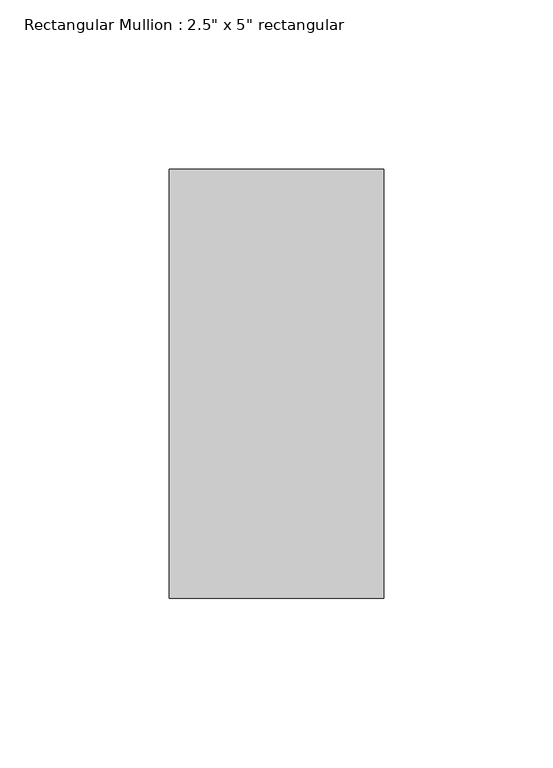
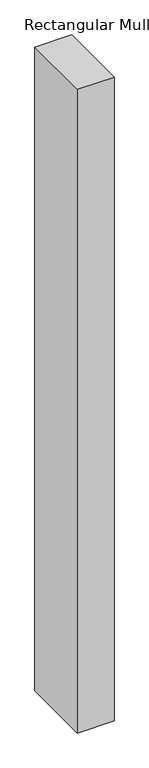
"""IFC4 building model written with IfcOpenShell, lengths in millimetres: member geometry."""

from ifc_helpers import new_model, si_unit, frame, origin, place, context, project, spatial, polyline, outline, extrude, source, transform, mapped, element, save


def member_3cc93373(model_context):
    return source(origin(), model_context, "Body", "SweptSolid", [
        extrude(outline(polyline([(0.0, 63.5), (0.0, -63.5), (-63.5, -63.5), (-63.5, 63.5), (0.0, 63.5)])), frame((0.0, 0.0, -1177.6398707), z_axis=(0.0, 0.0, 1.0), x_axis=(1.0, 0.0, 0.0)), (0.0, 0.0, 1.0), 1177.6398707),
    ])


if __name__ == "__main__":
    model = new_model("IFC4")
    model_context = context("Model", 3, world=origin())
    ifc_project = project(units=[si_unit("LENGTHUNIT", "METRE", prefix="MILLI")], contexts=[model_context])
    site = spatial("IfcSite", under=ifc_project)
    building = spatial("IfcBuilding", under=site)
    placement = place(None, origin())
    member_shape = member_3cc93373(model_context)
    element("IfcMember", 1, ObjectType="Rectangular Mullion : 2.5\" x 5\" rectangular", at=placement, inside=building, context=model_context, shape_type="MappedRepresentation", body=[
        mapped(member_shape, transform((0.0, 0.0, 0.0), x_axis=(1.0, 0.0, 0.0), y_axis=(0.0, 1.0, 0.0), z_axis=(0.0, 0.0, 1.0))),
    ])
    save(model, "model.ifc")

# Revit data of these elements
# Type "Rectangular Mullion : 2.5\" x 5\" rectangular"
#   built-in parameter 1007304 = 0.416667 (stored number, unit not read)
#   built-in parameter 1007301 = 0.104167 (stored number, unit not read)
#   built-in parameter 1007300 = 0.104167 (stored number, unit not read)
# Element 1 (IfcMember, "Rectangular Mullion : 2.5\" x 5\" rectangular")
#   Materials on its faces: "Aluminum"
# Materials
#   "Aluminum": class "Metal", colour RGB 247 247 247, transparency 0, Description = "Aluminum 6061", Cost = 0
